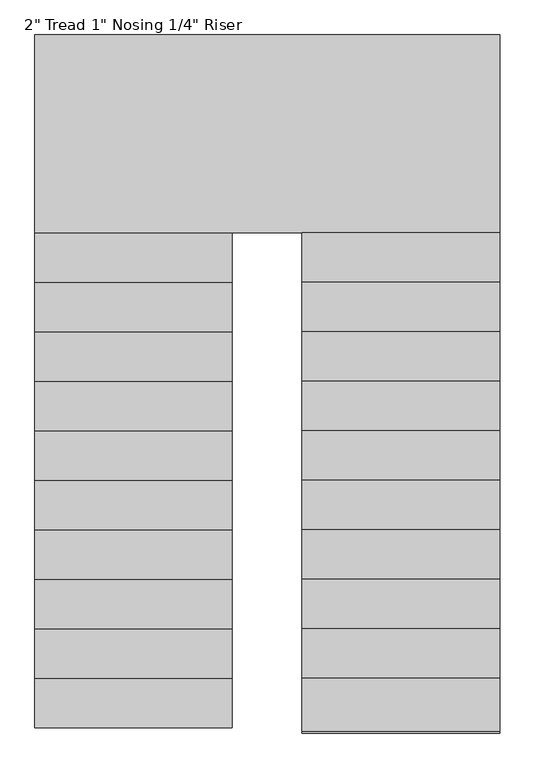
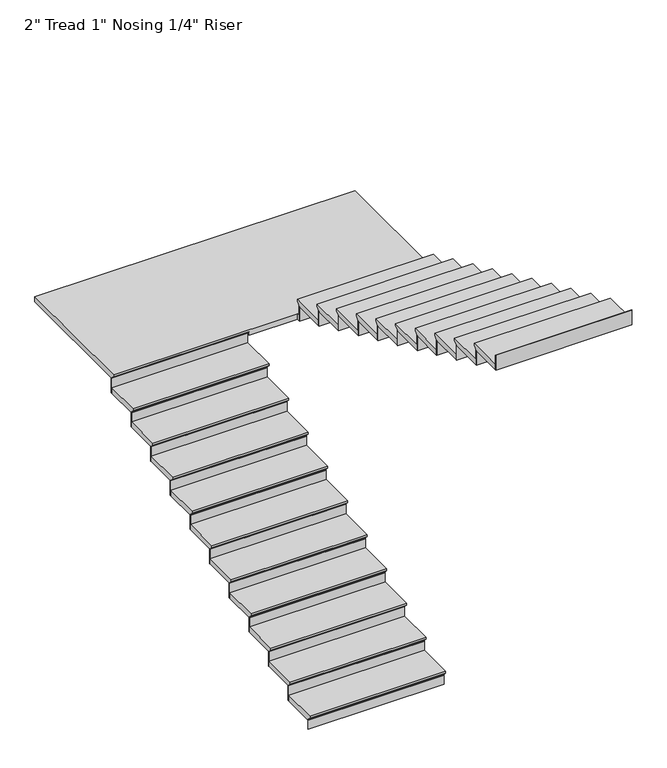
"""IFC4 building model written with IfcOpenShell, lengths in millimetres: stair flight geometry."""

from ifc_helpers import new_model, si_unit, origin, place, context, project, spatial, faceted_brep, source, transform, mapped, element, save


def stair_flight_8cbe8ac5(model_context):
    return source(origin(), model_context, "Body", "Brep", [
        faceted_brep([(-629.5987998, 3364.6067329, 32123.4954545), (-629.5987998, 3364.6067329, 32142.5454545), (-1845.5417538, 3364.6067329, 32142.5454545), (-1845.5417538, 3364.6067329, 32123.4954545), (-629.5987998, 3390.0067329, 32098.0954545), (-1845.5417538, 3390.0067329, 32098.0954545), (-629.5987998, 3694.8067329, 32142.5454545), (-1845.5417538, 3694.8067329, 32142.5454545), (-1845.5417538, 3390.0067329, 32091.7454545), (-1845.5417538, 3694.8067329, 32091.7454545), (-629.5987998, 3694.8067329, 32091.7454545), (-629.5987998, 3390.0067329, 32091.7454545)], [[[0, 1, 2, 3]], [[4, 0, 3, 5]], [[2, 1, 6, 7]], [[8, 9, 10, 11]], [[2, 7, 9, 8, 5, 3]], [[8, 11, 4, 5]], [[6, 1, 0, 4, 11, 10]], [[7, 6, 10, 9]]]),
        faceted_brep([(-629.5987998, 3390.0067329, 32091.7454545), (-629.5987998, 3390.0067329, 32004.0), (-629.5987998, 3396.3567329, 32004.0), (-629.5987998, 3396.3567329, 32091.7454545), (-1845.5417538, 3390.0067329, 32091.7454545), (-1845.5417538, 3396.3567329, 32091.7454545), (-1845.5417538, 3396.3567329, 32004.0), (-1845.5417538, 3390.0067329, 32004.0)], [[[0, 1, 2, 3]], [[4, 5, 6, 7]], [[1, 0, 4, 7]], [[2, 1, 7, 6]], [[3, 2, 6, 5]], [[0, 3, 5, 4]]]),
        faceted_brep([(-629.5987998, 3694.8067329, 32230.2909091), (-629.5987998, 3694.8067329, 32091.7454545), (-629.5987998, 3701.1567329, 32091.7454545), (-629.5987998, 3701.1567329, 32230.2909091), (-1845.5417538, 3694.8067329, 32230.2909091), (-1845.5417538, 3701.1567329, 32230.2909091), (-1845.5417538, 3701.1567329, 32091.7454545), (-1845.5417538, 3694.8067329, 32091.7454545)], [[[0, 1, 2, 3]], [[4, 5, 6, 7]], [[1, 0, 4, 7]], [[2, 1, 7, 6]], [[3, 2, 6, 5]], [[0, 3, 5, 4]]]),
        faceted_brep([(-1845.5417538, 3669.4067329, 32281.0909091), (-629.5987998, 3669.4067329, 32281.0909091), (-629.5987998, 3999.6067329, 32281.0909091), (-1845.5417538, 3999.6067329, 32281.0909091), (-1845.5417538, 3694.8067329, 32230.2909091), (-1845.5417538, 3999.6067329, 32230.2909091), (-629.5987998, 3999.6067329, 32230.2909091), (-629.5987998, 3694.8067329, 32230.2909091), (-1845.5417538, 3694.8067329, 32236.6409091), (-1845.5417538, 3669.4067329, 32262.0409091), (-629.5987998, 3694.8067329, 32236.6409091), (-629.5987998, 3669.4067329, 32262.0409091)], [[[0, 1, 2, 3]], [[4, 5, 6, 7]], [[0, 3, 5, 4, 8, 9]], [[4, 7, 10, 8]], [[2, 1, 11, 10, 7, 6]], [[3, 2, 6, 5]], [[11, 1, 0, 9]], [[10, 11, 9, 8]]]),
        faceted_brep([(-629.5987998, 3999.6067329, 32368.8363636), (-629.5987998, 3999.6067329, 32230.2909091), (-629.5987998, 4005.9567329, 32230.2909091), (-629.5987998, 4005.9567329, 32368.8363636), (-1845.5417538, 3999.6067329, 32368.8363636), (-1845.5417538, 4005.9567329, 32368.8363636), (-1845.5417538, 4005.9567329, 32230.2909091), (-1845.5417538, 3999.6067329, 32230.2909091)], [[[0, 1, 2, 3]], [[4, 5, 6, 7]], [[1, 0, 4, 7]], [[2, 1, 7, 6]], [[3, 2, 6, 5]], [[0, 3, 5, 4]]]),
        faceted_brep([(-1845.5417538, 3974.2067329, 32419.6363636), (-629.5987998, 3974.2067329, 32419.6363636), (-629.5987998, 4304.4067329, 32419.6363636), (-1845.5417538, 4304.4067329, 32419.6363636), (-1845.5417538, 3999.6067329, 32368.8363636), (-1845.5417538, 4304.4067329, 32368.8363636), (-629.5987998, 4304.4067329, 32368.8363636), (-629.5987998, 3999.6067329, 32368.8363636), (-1845.5417538, 3999.6067329, 32375.1863636), (-1845.5417538, 3974.2067329, 32400.5863636), (-629.5987998, 3999.6067329, 32375.1863636), (-629.5987998, 3974.2067329, 32400.5863636)], [[[0, 1, 2, 3]], [[4, 5, 6, 7]], [[0, 3, 5, 4, 8, 9]], [[4, 7, 10, 8]], [[2, 1, 11, 10, 7, 6]], [[3, 2, 6, 5]], [[11, 1, 0, 9]], [[10, 11, 9, 8]]]),
        faceted_brep([(-629.5987998, 4304.4067329, 32507.3818182), (-629.5987998, 4304.4067329, 32368.8363636), (-629.5987998, 4310.7567329, 32368.8363636), (-629.5987998, 4310.7567329, 32507.3818182), (-1845.5417538, 4304.4067329, 32507.3818182), (-1845.5417538, 4310.7567329, 32507.3818182), (-1845.5417538, 4310.7567329, 32368.8363636), (-1845.5417538, 4304.4067329, 32368.8363636)], [[[0, 1, 2, 3]], [[4, 5, 6, 7]], [[1, 0, 4, 7]], [[2, 1, 7, 6]], [[3, 2, 6, 5]], [[0, 3, 5, 4]]]),
        faceted_brep([(-1845.5417538, 4279.0067329, 32558.1818182), (-629.5987998, 4279.0067329, 32558.1818182), (-629.5987998, 4609.2067329, 32558.1818182), (-1845.5417538, 4609.2067329, 32558.1818182), (-1845.5417538, 4304.4067329, 32507.3818182), (-1845.5417538, 4609.2067329, 32507.3818182), (-629.5987998, 4609.2067329, 32507.3818182), (-629.5987998, 4304.4067329, 32507.3818182), (-1845.5417538, 4304.4067329, 32513.7318182), (-1845.5417538, 4279.0067329, 32539.1318182), (-629.5987998, 4304.4067329, 32513.7318182), (-629.5987998, 4279.0067329, 32539.1318182)], [[[0, 1, 2, 3]], [[4, 5, 6, 7]], [[0, 3, 5, 4, 8, 9]], [[4, 7, 10, 8]], [[2, 1, 11, 10, 7, 6]], [[3, 2, 6, 5]], [[11, 1, 0, 9]], [[10, 11, 9, 8]]]),
        faceted_brep([(-629.5987998, 4609.2067329, 32645.9272727), (-629.5987998, 4609.2067329, 32507.3818182), (-629.5987998, 4615.5567329, 32507.3818182), (-629.5987998, 4615.5567329, 32645.9272727), (-1845.5417538, 4609.2067329, 32645.9272727), (-1845.5417538, 4615.5567329, 32645.9272727), (-1845.5417538, 4615.5567329, 32507.3818182), (-1845.5417538, 4609.2067329, 32507.3818182)], [[[0, 1, 2, 3]], [[4, 5, 6, 7]], [[1, 0, 4, 7]], [[2, 1, 7, 6]], [[3, 2, 6, 5]], [[0, 3, 5, 4]]]),
        faceted_brep([(-1845.5417538, 4583.8067329, 32696.7272727), (-629.5987998, 4583.8067329, 32696.7272727), (-629.5987998, 4914.0067329, 32696.7272727), (-1845.5417538, 4914.0067329, 32696.7272727), (-1845.5417538, 4609.2067329, 32645.9272727), (-1845.5417538, 4914.0067329, 32645.9272727), (-629.5987998, 4914.0067329, 32645.9272727), (-629.5987998, 4609.2067329, 32645.9272727), (-1845.5417538, 4609.2067329, 32652.2772727), (-1845.5417538, 4583.8067329, 32677.6772727), (-629.5987998, 4609.2067329, 32652.2772727), (-629.5987998, 4583.8067329, 32677.6772727)], [[[0, 1, 2, 3]], [[4, 5, 6, 7]], [[0, 3, 5, 4, 8, 9]], [[4, 7, 10, 8]], [[2, 1, 11, 10, 7, 6]], [[3, 2, 6, 5]], [[11, 1, 0, 9]], [[10, 11, 9, 8]]]),
        faceted_brep([(-629.5987998, 4914.0067329, 32784.4727273), (-629.5987998, 4914.0067329, 32645.9272727), (-629.5987998, 4920.3567329, 32645.9272727), (-629.5987998, 4920.3567329, 32784.4727273), (-1845.5417538, 4914.0067329, 32784.4727273), (-1845.5417538, 4920.3567329, 32784.4727273), (-1845.5417538, 4920.3567329, 32645.9272727), (-1845.5417538, 4914.0067329, 32645.9272727)], [[[0, 1, 2, 3]], [[4, 5, 6, 7]], [[1, 0, 4, 7]], [[2, 1, 7, 6]], [[3, 2, 6, 5]], [[0, 3, 5, 4]]]),
        faceted_brep([(-1845.5417538, 4888.6067329, 32835.2727273), (-629.5987998, 4888.6067329, 32835.2727273), (-629.5987998, 5218.8067329, 32835.2727273), (-1845.5417538, 5218.8067329, 32835.2727273), (-1845.5417538, 4914.0067329, 32784.4727273), (-1845.5417538, 5218.8067329, 32784.4727273), (-629.5987998, 5218.8067329, 32784.4727273), (-629.5987998, 4914.0067329, 32784.4727273), (-1845.5417538, 4914.0067329, 32790.8227273), (-1845.5417538, 4888.6067329, 32816.2227273), (-629.5987998, 4914.0067329, 32790.8227273), (-629.5987998, 4888.6067329, 32816.2227273)], [[[0, 1, 2, 3]], [[4, 5, 6, 7]], [[0, 3, 5, 4, 8, 9]], [[4, 7, 10, 8]], [[2, 1, 11, 10, 7, 6]], [[3, 2, 6, 5]], [[11, 1, 0, 9]], [[10, 11, 9, 8]]]),
        faceted_brep([(-629.5987998, 5218.8067329, 32923.0181818), (-629.5987998, 5218.8067329, 32784.4727273), (-629.5987998, 5225.1567329, 32784.4727273), (-629.5987998, 5225.1567329, 32923.0181818), (-1845.5417538, 5218.8067329, 32923.0181818), (-1845.5417538, 5225.1567329, 32923.0181818), (-1845.5417538, 5225.1567329, 32784.4727273), (-1845.5417538, 5218.8067329, 32784.4727273)], [[[0, 1, 2, 3]], [[4, 5, 6, 7]], [[1, 0, 4, 7]], [[2, 1, 7, 6]], [[3, 2, 6, 5]], [[0, 3, 5, 4]]]),
        faceted_brep([(-1845.5417538, 5193.4067329, 32973.8181818), (-629.5987998, 5193.4067329, 32973.8181818), (-629.5987998, 5523.6067329, 32973.8181818), (-1845.5417538, 5523.6067329, 32973.8181818), (-1845.5417538, 5218.8067329, 32923.0181818), (-1845.5417538, 5523.6067329, 32923.0181818), (-629.5987998, 5523.6067329, 32923.0181818), (-629.5987998, 5218.8067329, 32923.0181818), (-1845.5417538, 5218.8067329, 32929.3681818), (-1845.5417538, 5193.4067329, 32954.7681818), (-629.5987998, 5218.8067329, 32929.3681818), (-629.5987998, 5193.4067329, 32954.7681818)], [[[0, 1, 2, 3]], [[4, 5, 6, 7]], [[0, 3, 5, 4, 8, 9]], [[4, 7, 10, 8]], [[2, 1, 11, 10, 7, 6]], [[3, 2, 6, 5]], [[11, 1, 0, 9]], [[10, 11, 9, 8]]]),
        faceted_brep([(-629.5987998, 5523.6067329, 33061.5636364), (-629.5987998, 5523.6067329, 32923.0181818), (-629.5987998, 5529.9567329, 32923.0181818), (-629.5987998, 5529.9567329, 33061.5636364), (-1845.5417538, 5523.6067329, 33061.5636364), (-1845.5417538, 5529.9567329, 33061.5636364), (-1845.5417538, 5529.9567329, 32923.0181818), (-1845.5417538, 5523.6067329, 32923.0181818)], [[[0, 1, 2, 3]], [[4, 5, 6, 7]], [[1, 0, 4, 7]], [[2, 1, 7, 6]], [[3, 2, 6, 5]], [[0, 3, 5, 4]]]),
        faceted_brep([(-1845.5417538, 5498.2067329, 33112.3636364), (-629.5987998, 5498.2067329, 33112.3636364), (-629.5987998, 5828.4067329, 33112.3636364), (-1845.5417538, 5828.4067329, 33112.3636364), (-1845.5417538, 5523.6067329, 33061.5636364), (-1845.5417538, 5828.4067329, 33061.5636364), (-629.5987998, 5828.4067329, 33061.5636364), (-629.5987998, 5523.6067329, 33061.5636364), (-1845.5417538, 5523.6067329, 33067.9136364), (-1845.5417538, 5498.2067329, 33093.3136364), (-629.5987998, 5523.6067329, 33067.9136364), (-629.5987998, 5498.2067329, 33093.3136364)], [[[0, 1, 2, 3]], [[4, 5, 6, 7]], [[0, 3, 5, 4, 8, 9]], [[4, 7, 10, 8]], [[2, 1, 11, 10, 7, 6]], [[3, 2, 6, 5]], [[11, 1, 0, 9]], [[10, 11, 9, 8]]]),
        faceted_brep([(-629.5987998, 5828.4067329, 33200.1090909), (-629.5987998, 5828.4067329, 33061.5636364), (-629.5987998, 5834.7567329, 33061.5636364), (-629.5987998, 5834.7567329, 33200.1090909), (-1845.5417538, 5828.4067329, 33200.1090909), (-1845.5417538, 5834.7567329, 33200.1090909), (-1845.5417538, 5834.7567329, 33061.5636364), (-1845.5417538, 5828.4067329, 33061.5636364)], [[[0, 1, 2, 3]], [[4, 5, 6, 7]], [[1, 0, 4, 7]], [[2, 1, 7, 6]], [[3, 2, 6, 5]], [[0, 3, 5, 4]]]),
        faceted_brep([(-1845.5417538, 5803.0067329, 33250.9090909), (-629.5987998, 5803.0067329, 33250.9090909), (-629.5987998, 6133.2067329, 33250.9090909), (-1845.5417538, 6133.2067329, 33250.9090909), (-1845.5417538, 5828.4067329, 33200.1090909), (-1845.5417538, 6133.2067329, 33200.1090909), (-629.5987998, 6133.2067329, 33200.1090909), (-629.5987998, 5828.4067329, 33200.1090909), (-1845.5417538, 5828.4067329, 33206.4590909), (-1845.5417538, 5803.0067329, 33231.8590909), (-629.5987998, 5828.4067329, 33206.4590909), (-629.5987998, 5803.0067329, 33231.8590909)], [[[0, 1, 2, 3]], [[4, 5, 6, 7]], [[0, 3, 5, 4, 8, 9]], [[4, 7, 10, 8]], [[2, 1, 11, 10, 7, 6]], [[3, 2, 6, 5]], [[11, 1, 0, 9]], [[10, 11, 9, 8]]]),
        faceted_brep([(-629.5987998, 6133.2067329, 33338.6545455), (-629.5987998, 6133.2067329, 33200.1090909), (-629.5987998, 6139.5567329, 33200.1090909), (-629.5987998, 6139.5567329, 33338.6545455), (-1845.5417538, 6133.2067329, 33338.6545455), (-1845.5417538, 6139.5567329, 33338.6545455), (-1845.5417538, 6139.5567329, 33200.1090909), (-1845.5417538, 6133.2067329, 33200.1090909)], [[[0, 1, 2, 3]], [[4, 5, 6, 7]], [[1, 0, 4, 7]], [[2, 1, 7, 6]], [[3, 2, 6, 5]], [[0, 3, 5, 4]]]),
        faceted_brep([(-1845.5417538, 6107.8067329, 33389.4545455), (-629.5987998, 6107.8067329, 33389.4545455), (-629.5987998, 6438.0067329, 33389.4545455), (-1845.5417538, 6438.0067329, 33389.4545455), (-1845.5417538, 6133.2067329, 33338.6545455), (-1845.5417538, 6438.0067329, 33338.6545455), (-629.5987998, 6438.0067329, 33338.6545455), (-629.5987998, 6133.2067329, 33338.6545455), (-1845.5417538, 6133.2067329, 33345.0045455), (-1845.5417538, 6107.8067329, 33370.4045455), (-629.5987998, 6133.2067329, 33345.0045455), (-629.5987998, 6107.8067329, 33370.4045455)], [[[0, 1, 2, 3]], [[4, 5, 6, 7]], [[0, 3, 5, 4, 8, 9]], [[4, 7, 10, 8]], [[2, 1, 11, 10, 7, 6]], [[3, 2, 6, 5]], [[11, 1, 0, 9]], [[10, 11, 9, 8]]]),
        faceted_brep([(-629.5987998, 6438.0067329, 33477.2), (-629.5987998, 6438.0067329, 33338.6545455), (-629.5987998, 6444.3567329, 33338.6545455), (-629.5987998, 6444.3567329, 33477.2), (-1845.5417538, 6438.0067329, 33477.2), (-1845.5417538, 6444.3567329, 33477.2), (-1845.5417538, 6444.3567329, 33338.6545455), (-1845.5417538, 6438.0067329, 33338.6545455)], [[[0, 1, 2, 3]], [[4, 5, 6, 7]], [[1, 0, 4, 7]], [[2, 1, 7, 6]], [[3, 2, 6, 5]], [[0, 3, 5, 4]]]),
        faceted_brep([(1021.4012085, 6387.2067329, 33528.0), (1021.4012085, 7631.8067329, 33528.0), (-1845.5417538, 7631.8067329, 33528.0), (-1845.5417538, 6412.6067329, 33528.0), (-197.7987915, 6412.6067329, 33528.0), (-197.7987915, 6387.2067329, 33528.0), (1021.4012085, 7631.8067329, 33477.2), (1021.4012085, 6387.2067329, 33477.2), (-197.7987915, 6387.2067329, 33477.2), (-197.7987915, 6412.6067329, 33477.2), (-629.5987998, 6412.6067329, 33477.2), (-629.5987998, 6438.0067329, 33477.2), (-1845.5417538, 6438.0067329, 33477.2), (-1845.5417538, 7631.8067329, 33477.2), (-629.5987998, 6438.0067329, 33483.55), (-1845.5417538, 6438.0067329, 33483.55), (-1845.5417538, 6412.6067329, 33508.95), (-629.5987998, 6412.6067329, 33508.95)], [[[0, 1, 2, 3, 4, 5]], [[6, 7, 8, 9, 10, 11, 12, 13]], [[1, 0, 7, 6]], [[2, 1, 6, 13]], [[12, 11, 14, 15]], [[4, 3, 16, 17, 10, 9]], [[5, 4, 9, 8]], [[0, 5, 8, 7]], [[16, 15, 14, 17]], [[3, 2, 13, 12, 15, 16]], [[11, 10, 17, 14]]]),
        faceted_brep([(-197.7987915, 6387.2067329, 33615.7454545), (-197.7987915, 6387.2067329, 33477.2), (-197.7987915, 6380.8567329, 33477.2), (-197.7987915, 6380.8567329, 33615.7454545), (1021.4012085, 6387.2067329, 33615.7454545), (1021.4012085, 6380.8567329, 33615.7454545), (1021.4012085, 6380.8567329, 33477.2), (1021.4012085, 6387.2067329, 33477.2)], [[[0, 1, 2, 3]], [[4, 5, 6, 7]], [[1, 0, 4, 7]], [[2, 1, 7, 6]], [[3, 2, 6, 5]], [[0, 3, 5, 4]]]),
        faceted_brep([(1021.4012085, 6412.6067329, 33666.5454545), (-197.7987915, 6412.6067329, 33666.5454545), (-197.7987915, 6082.4067329, 33666.5454545), (1021.4012085, 6082.4067329, 33666.5454545), (1021.4012085, 6387.2067329, 33615.7454545), (1021.4012085, 6082.4067329, 33615.7454545), (-197.7987915, 6082.4067329, 33615.7454545), (-197.7987915, 6387.2067329, 33615.7454545), (1021.4012085, 6387.2067329, 33622.0954545), (1021.4012085, 6412.6067329, 33647.4954545), (-197.7987915, 6387.2067329, 33622.0954545), (-197.7987915, 6412.6067329, 33647.4954545)], [[[0, 1, 2, 3]], [[4, 5, 6, 7]], [[0, 3, 5, 4, 8, 9]], [[4, 7, 10, 8]], [[2, 1, 11, 10, 7, 6]], [[3, 2, 6, 5]], [[11, 1, 0, 9]], [[10, 11, 9, 8]]]),
        faceted_brep([(-197.7987915, 6082.4067329, 33754.2909091), (-197.7987915, 6082.4067329, 33615.7454545), (-197.7987915, 6076.0567329, 33615.7454545), (-197.7987915, 6076.0567329, 33754.2909091), (1021.4012085, 6082.4067329, 33754.2909091), (1021.4012085, 6076.0567329, 33754.2909091), (1021.4012085, 6076.0567329, 33615.7454545), (1021.4012085, 6082.4067329, 33615.7454545)], [[[0, 1, 2, 3]], [[4, 5, 6, 7]], [[1, 0, 4, 7]], [[2, 1, 7, 6]], [[3, 2, 6, 5]], [[0, 3, 5, 4]]]),
        faceted_brep([(1021.4012085, 6107.8067329, 33805.0909091), (-197.7987915, 6107.8067329, 33805.0909091), (-197.7987915, 5777.6067329, 33805.0909091), (1021.4012085, 5777.6067329, 33805.0909091), (1021.4012085, 6082.4067329, 33754.2909091), (1021.4012085, 5777.6067329, 33754.2909091), (-197.7987915, 5777.6067329, 33754.2909091), (-197.7987915, 6082.4067329, 33754.2909091), (1021.4012085, 6082.4067329, 33760.6409091), (1021.4012085, 6107.8067329, 33786.0409091), (-197.7987915, 6082.4067329, 33760.6409091), (-197.7987915, 6107.8067329, 33786.0409091)], [[[0, 1, 2, 3]], [[4, 5, 6, 7]], [[0, 3, 5, 4, 8, 9]], [[4, 7, 10, 8]], [[2, 1, 11, 10, 7, 6]], [[3, 2, 6, 5]], [[11, 1, 0, 9]], [[10, 11, 9, 8]]]),
        faceted_brep([(-197.7987915, 5777.6067329, 33892.8363636), (-197.7987915, 5777.6067329, 33754.2909091), (-197.7987915, 5771.2567329, 33754.2909091), (-197.7987915, 5771.2567329, 33892.8363636), (1021.4012085, 5777.6067329, 33892.8363636), (1021.4012085, 5771.2567329, 33892.8363636), (1021.4012085, 5771.2567329, 33754.2909091), (1021.4012085, 5777.6067329, 33754.2909091)], [[[0, 1, 2, 3]], [[4, 5, 6, 7]], [[1, 0, 4, 7]], [[2, 1, 7, 6]], [[3, 2, 6, 5]], [[0, 3, 5, 4]]]),
        faceted_brep([(1021.4012085, 5803.0067329, 33943.6363636), (-197.7987915, 5803.0067329, 33943.6363636), (-197.7987915, 5472.8067329, 33943.6363636), (1021.4012085, 5472.8067329, 33943.6363636), (1021.4012085, 5777.6067329, 33892.8363636), (1021.4012085, 5472.8067329, 33892.8363636), (-197.7987915, 5472.8067329, 33892.8363636), (-197.7987915, 5777.6067329, 33892.8363636), (1021.4012085, 5777.6067329, 33899.1863636), (1021.4012085, 5803.0067329, 33924.5863636), (-197.7987915, 5777.6067329, 33899.1863636), (-197.7987915, 5803.0067329, 33924.5863636)], [[[0, 1, 2, 3]], [[4, 5, 6, 7]], [[0, 3, 5, 4, 8, 9]], [[4, 7, 10, 8]], [[2, 1, 11, 10, 7, 6]], [[3, 2, 6, 5]], [[11, 1, 0, 9]], [[10, 11, 9, 8]]]),
        faceted_brep([(-197.7987915, 5472.8067329, 34031.3818182), (-197.7987915, 5472.8067329, 33892.8363636), (-197.7987915, 5466.4567329, 33892.8363636), (-197.7987915, 5466.4567329, 34031.3818182), (1021.4012085, 5472.8067329, 34031.3818182), (1021.4012085, 5466.4567329, 34031.3818182), (1021.4012085, 5466.4567329, 33892.8363636), (1021.4012085, 5472.8067329, 33892.8363636)], [[[0, 1, 2, 3]], [[4, 5, 6, 7]], [[1, 0, 4, 7]], [[2, 1, 7, 6]], [[3, 2, 6, 5]], [[0, 3, 5, 4]]]),
        faceted_brep([(1021.4012085, 5498.2067329, 34082.1818182), (-197.7987915, 5498.2067329, 34082.1818182), (-197.7987915, 5168.0067329, 34082.1818182), (1021.4012085, 5168.0067329, 34082.1818182), (1021.4012085, 5472.8067329, 34031.3818182), (1021.4012085, 5168.0067329, 34031.3818182), (-197.7987915, 5168.0067329, 34031.3818182), (-197.7987915, 5472.8067329, 34031.3818182), (1021.4012085, 5472.8067329, 34037.7318182), (1021.4012085, 5498.2067329, 34063.1318182), (-197.7987915, 5472.8067329, 34037.7318182), (-197.7987915, 5498.2067329, 34063.1318182)], [[[0, 1, 2, 3]], [[4, 5, 6, 7]], [[0, 3, 5, 4, 8, 9]], [[4, 7, 10, 8]], [[2, 1, 11, 10, 7, 6]], [[3, 2, 6, 5]], [[11, 1, 0, 9]], [[10, 11, 9, 8]]]),
        faceted_brep([(-197.7987915, 5168.0067329, 34169.9272727), (-197.7987915, 5168.0067329, 34031.3818182), (-197.7987915, 5161.6567329, 34031.3818182), (-197.7987915, 5161.6567329, 34169.9272727), (1021.4012085, 5168.0067329, 34169.9272727), (1021.4012085, 5161.6567329, 34169.9272727), (1021.4012085, 5161.6567329, 34031.3818182), (1021.4012085, 5168.0067329, 34031.3818182)], [[[0, 1, 2, 3]], [[4, 5, 6, 7]], [[1, 0, 4, 7]], [[2, 1, 7, 6]], [[3, 2, 6, 5]], [[0, 3, 5, 4]]]),
        faceted_brep([(1021.4012085, 5193.4067329, 34220.7272727), (-197.7987915, 5193.4067329, 34220.7272727), (-197.7987915, 4863.2067329, 34220.7272727), (1021.4012085, 4863.2067329, 34220.7272727), (1021.4012085, 5168.0067329, 34169.9272727), (1021.4012085, 4863.2067329, 34169.9272727), (-197.7987915, 4863.2067329, 34169.9272727), (-197.7987915, 5168.0067329, 34169.9272727), (1021.4012085, 5168.0067329, 34176.2772727), (1021.4012085, 5193.4067329, 34201.6772727), (-197.7987915, 5168.0067329, 34176.2772727), (-197.7987915, 5193.4067329, 34201.6772727)], [[[0, 1, 2, 3]], [[4, 5, 6, 7]], [[0, 3, 5, 4, 8, 9]], [[4, 7, 10, 8]], [[2, 1, 11, 10, 7, 6]], [[3, 2, 6, 5]], [[11, 1, 0, 9]], [[10, 11, 9, 8]]]),
        faceted_brep([(-197.7987915, 4863.2067329, 34308.4727273), (-197.7987915, 4863.2067329, 34169.9272727), (-197.7987915, 4856.8567329, 34169.9272727), (-197.7987915, 4856.8567329, 34308.4727273), (1021.4012085, 4863.2067329, 34308.4727273), (1021.4012085, 4856.8567329, 34308.4727273), (1021.4012085, 4856.8567329, 34169.9272727), (1021.4012085, 4863.2067329, 34169.9272727)], [[[0, 1, 2, 3]], [[4, 5, 6, 7]], [[1, 0, 4, 7]], [[2, 1, 7, 6]], [[3, 2, 6, 5]], [[0, 3, 5, 4]]]),
        faceted_brep([(1021.4012085, 4888.6067329, 34359.2727273), (-197.7987915, 4888.6067329, 34359.2727273), (-197.7987915, 4558.4067329, 34359.2727273), (1021.4012085, 4558.4067329, 34359.2727273), (1021.4012085, 4863.2067329, 34308.4727273), (1021.4012085, 4558.4067329, 34308.4727273), (-197.7987915, 4558.4067329, 34308.4727273), (-197.7987915, 4863.2067329, 34308.4727273), (1021.4012085, 4863.2067329, 34314.8227273), (1021.4012085, 4888.6067329, 34340.2227273), (-197.7987915, 4863.2067329, 34314.8227273), (-197.7987915, 4888.6067329, 34340.2227273)], [[[0, 1, 2, 3]], [[4, 5, 6, 7]], [[0, 3, 5, 4, 8, 9]], [[4, 7, 10, 8]], [[2, 1, 11, 10, 7, 6]], [[3, 2, 6, 5]], [[11, 1, 0, 9]], [[10, 11, 9, 8]]]),
        faceted_brep([(-197.7987915, 4558.4067329, 34447.0181818), (-197.7987915, 4558.4067329, 34308.4727273), (-197.7987915, 4552.0567329, 34308.4727273), (-197.7987915, 4552.0567329, 34447.0181818), (1021.4012085, 4558.4067329, 34447.0181818), (1021.4012085, 4552.0567329, 34447.0181818), (1021.4012085, 4552.0567329, 34308.4727273), (1021.4012085, 4558.4067329, 34308.4727273)], [[[0, 1, 2, 3]], [[4, 5, 6, 7]], [[1, 0, 4, 7]], [[2, 1, 7, 6]], [[3, 2, 6, 5]], [[0, 3, 5, 4]]]),
        faceted_brep([(1021.4012085, 4583.8067329, 34497.8181818), (-197.7987915, 4583.8067329, 34497.8181818), (-197.7987915, 4253.6067329, 34497.8181818), (1021.4012085, 4253.6067329, 34497.8181818), (1021.4012085, 4558.4067329, 34447.0181818), (1021.4012085, 4253.6067329, 34447.0181818), (-197.7987915, 4253.6067329, 34447.0181818), (-197.7987915, 4558.4067329, 34447.0181818), (1021.4012085, 4558.4067329, 34453.3681818), (1021.4012085, 4583.8067329, 34478.7681818), (-197.7987915, 4558.4067329, 34453.3681818), (-197.7987915, 4583.8067329, 34478.7681818)], [[[0, 1, 2, 3]], [[4, 5, 6, 7]], [[0, 3, 5, 4, 8, 9]], [[4, 7, 10, 8]], [[2, 1, 11, 10, 7, 6]], [[3, 2, 6, 5]], [[11, 1, 0, 9]], [[10, 11, 9, 8]]]),
        faceted_brep([(-197.7987915, 4253.6067329, 34585.5636364), (-197.7987915, 4253.6067329, 34447.0181818), (-197.7987915, 4247.2567329, 34447.0181818), (-197.7987915, 4247.2567329, 34585.5636364), (1021.4012085, 4253.6067329, 34585.5636364), (1021.4012085, 4247.2567329, 34585.5636364), (1021.4012085, 4247.2567329, 34447.0181818), (1021.4012085, 4253.6067329, 34447.0181818)], [[[0, 1, 2, 3]], [[4, 5, 6, 7]], [[1, 0, 4, 7]], [[2, 1, 7, 6]], [[3, 2, 6, 5]], [[0, 3, 5, 4]]]),
        faceted_brep([(1021.4012085, 4279.0067329, 34636.3636364), (-197.7987915, 4279.0067329, 34636.3636364), (-197.7987915, 3948.8067329, 34636.3636364), (1021.4012085, 3948.8067329, 34636.3636364), (1021.4012085, 4253.6067329, 34585.5636364), (1021.4012085, 3948.8067329, 34585.5636364), (-197.7987915, 3948.8067329, 34585.5636364), (-197.7987915, 4253.6067329, 34585.5636364), (1021.4012085, 4253.6067329, 34591.9136364), (1021.4012085, 4279.0067329, 34617.3136364), (-197.7987915, 4253.6067329, 34591.9136364), (-197.7987915, 4279.0067329, 34617.3136364)], [[[0, 1, 2, 3]], [[4, 5, 6, 7]], [[0, 3, 5, 4, 8, 9]], [[4, 7, 10, 8]], [[2, 1, 11, 10, 7, 6]], [[3, 2, 6, 5]], [[11, 1, 0, 9]], [[10, 11, 9, 8]]]),
        faceted_brep([(-197.7987915, 3948.8067329, 34724.1090909), (-197.7987915, 3948.8067329, 34585.5636364), (-197.7987915, 3942.4567329, 34585.5636364), (-197.7987915, 3942.4567329, 34724.1090909), (1021.4012085, 3948.8067329, 34724.1090909), (1021.4012085, 3942.4567329, 34724.1090909), (1021.4012085, 3942.4567329, 34585.5636364), (1021.4012085, 3948.8067329, 34585.5636364)], [[[0, 1, 2, 3]], [[4, 5, 6, 7]], [[1, 0, 4, 7]], [[2, 1, 7, 6]], [[3, 2, 6, 5]], [[0, 3, 5, 4]]]),
        faceted_brep([(1021.4012085, 3974.2067329, 34774.9090909), (-197.7987915, 3974.2067329, 34774.9090909), (-197.7987915, 3644.0067329, 34774.9090909), (1021.4012085, 3644.0067329, 34774.9090909), (1021.4012085, 3948.8067329, 34724.1090909), (1021.4012085, 3644.0067329, 34724.1090909), (-197.7987915, 3644.0067329, 34724.1090909), (-197.7987915, 3948.8067329, 34724.1090909), (1021.4012085, 3948.8067329, 34730.4590909), (1021.4012085, 3974.2067329, 34755.8590909), (-197.7987915, 3948.8067329, 34730.4590909), (-197.7987915, 3974.2067329, 34755.8590909)], [[[0, 1, 2, 3]], [[4, 5, 6, 7]], [[0, 3, 5, 4, 8, 9]], [[4, 7, 10, 8]], [[2, 1, 11, 10, 7, 6]], [[3, 2, 6, 5]], [[11, 1, 0, 9]], [[10, 11, 9, 8]]]),
        faceted_brep([(-197.7987915, 3644.0067329, 34862.6545455), (-197.7987915, 3644.0067329, 34724.1090909), (-197.7987915, 3637.6567329, 34724.1090909), (-197.7987915, 3637.6567329, 34862.6545455), (1021.4012085, 3644.0067329, 34862.6545455), (1021.4012085, 3637.6567329, 34862.6545455), (1021.4012085, 3637.6567329, 34724.1090909), (1021.4012085, 3644.0067329, 34724.1090909)], [[[0, 1, 2, 3]], [[4, 5, 6, 7]], [[1, 0, 4, 7]], [[2, 1, 7, 6]], [[3, 2, 6, 5]], [[0, 3, 5, 4]]]),
        faceted_brep([(-197.7987915, 3339.2067329, 35001.2), (-197.7987915, 3339.2067329, 34862.6545455), (-197.7987915, 3332.8567329, 34862.6545455), (-197.7987915, 3332.8567329, 35001.2), (1021.4012085, 3339.2067329, 35001.2), (1021.4012085, 3332.8567329, 35001.2), (1021.4012085, 3332.8567329, 34862.6545455), (1021.4012085, 3339.2067329, 34862.6545455)], [[[0, 1, 2, 3]], [[4, 5, 6, 7]], [[1, 0, 4, 7]], [[2, 1, 7, 6]], [[3, 2, 6, 5]], [[0, 3, 5, 4]]]),
        faceted_brep([(1021.4012085, 3669.4067329, 34913.4545455), (-197.7987915, 3669.4067329, 34913.4545455), (-197.7987915, 3339.2067329, 34913.4545455), (1021.4012085, 3339.2067329, 34913.4545455), (1021.4012085, 3644.0067329, 34862.6545455), (1021.4012085, 3339.2067329, 34862.6545455), (-197.7987915, 3339.2067329, 34862.6545455), (-197.7987915, 3644.0067329, 34862.6545455), (1021.4012085, 3644.0067329, 34869.0045455), (1021.4012085, 3669.4067329, 34894.4045455), (-197.7987915, 3644.0067329, 34869.0045455), (-197.7987915, 3669.4067329, 34894.4045455)], [[[0, 1, 2, 3]], [[4, 5, 6, 7]], [[0, 3, 5, 4, 8, 9]], [[4, 7, 10, 8]], [[2, 1, 11, 10, 7, 6]], [[3, 2, 6, 5]], [[11, 1, 0, 9]], [[10, 11, 9, 8]]]),
    ])


if __name__ == "__main__":
    model = new_model("IFC4")
    model_context = context("Model", 3, world=origin())
    ifc_project = project(units=[si_unit("LENGTHUNIT", "METRE", prefix="MILLI")], contexts=[model_context])
    site = spatial("IfcSite", under=ifc_project)
    building = spatial("IfcBuilding", under=site)
    placement = place(None, origin())
    stair_flight_shape = stair_flight_8cbe8ac5(model_context)
    element("IfcStairFlight", 1, ObjectType="2\" Tread 1\" Nosing 1/4\" Riser", at=placement, inside=building, context=model_context, shape_type="MappedRepresentation", body=[
        mapped(stair_flight_shape, transform((0.0, 0.0, 0.0), x_axis=(1.0, 0.0, 0.0), y_axis=(0.0, 1.0, 0.0), z_axis=(0.0, 0.0, 1.0))),
    ])
    save(model, "model.ifc")
